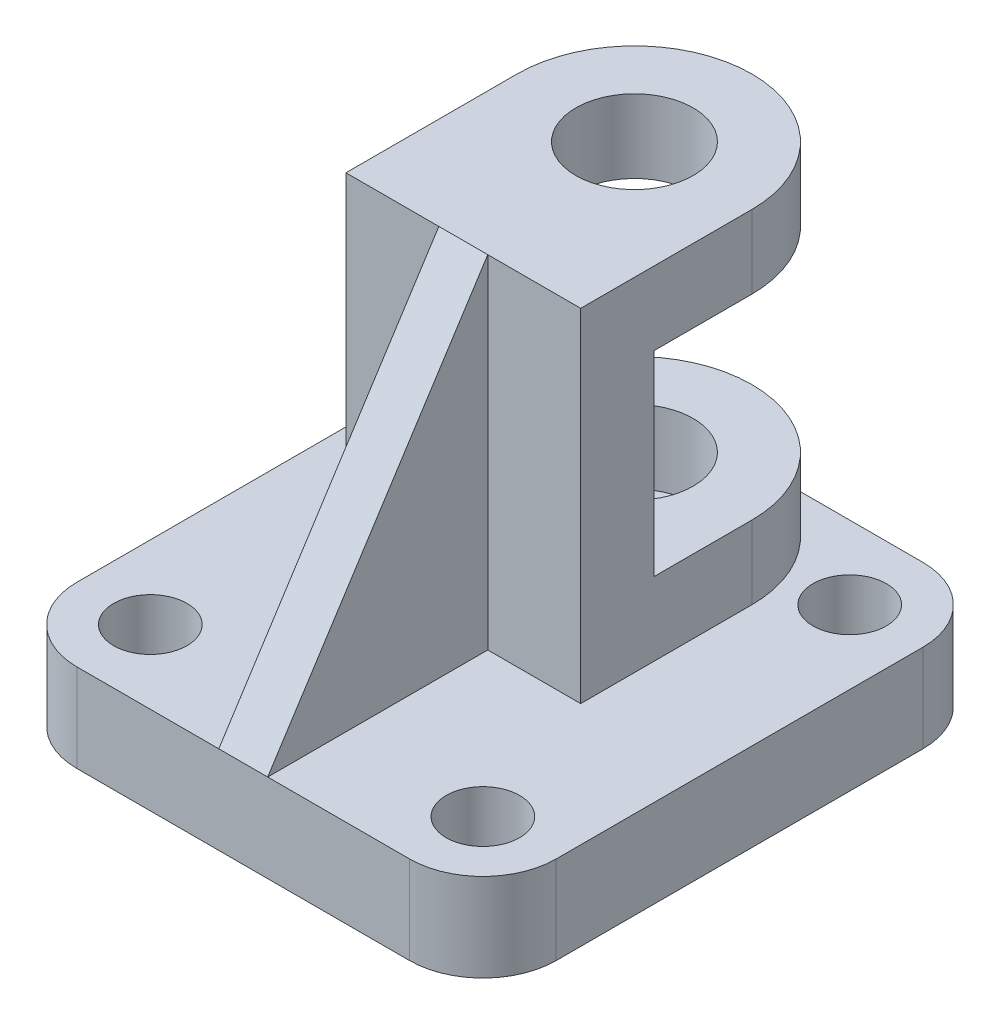
ISO-10303-21;
HEADER;
FILE_DESCRIPTION(('STEP AP214'),'2;1');
FILE_NAME('part.step','',(''),(''),'','','');
FILE_SCHEMA(('AUTOMOTIVE_DESIGN { 1 0 10303 214 1 1 1 1 }'));
ENDSEC;
DATA;
#1=APPLICATION_CONTEXT('core data for automotive mechanical design processes');
#2=APPLICATION_PROTOCOL_DEFINITION('international standard','automotive_design',2000,#1);
#3=PRODUCT_CONTEXT('',#1,'mechanical');
#4=PRODUCT('Part','Part','',(#3));
#5=PRODUCT_RELATED_PRODUCT_CATEGORY('part','',(#4));
#6=PRODUCT_DEFINITION_FORMATION('','',#4);
#7=PRODUCT_DEFINITION_CONTEXT('part definition',#1,'design');
#8=PRODUCT_DEFINITION('design','',#6,#7);
#9=PRODUCT_DEFINITION_SHAPE('','',#8);
#10=(LENGTH_UNIT() NAMED_UNIT(*) SI_UNIT(.MILLI.,.METRE.));
#11=(NAMED_UNIT(*) PLANE_ANGLE_UNIT() SI_UNIT($,.RADIAN.));
#12=(NAMED_UNIT(*) SI_UNIT($,.STERADIAN.) SOLID_ANGLE_UNIT());
#13=UNCERTAINTY_MEASURE_WITH_UNIT(LENGTH_MEASURE(1.E-05),#10,'distance_accuracy_value','');
#14=(GEOMETRIC_REPRESENTATION_CONTEXT(3) GLOBAL_UNCERTAINTY_ASSIGNED_CONTEXT((#13)) GLOBAL_UNIT_ASSIGNED_CONTEXT((#10,
#11,#12)) REPRESENTATION_CONTEXT('',''));
#15=CARTESIAN_POINT('',(0.,0.,0.));
#16=DIRECTION('',(0.,0.,1.));
#17=DIRECTION('',(1.,0.,0.));
#18=AXIS2_PLACEMENT_3D('',#15,#16,#17);
#19=CARTESIAN_POINT('',(0.,0.,7.5));
#20=DIRECTION('',(0.,0.,-1.));
#21=DIRECTION('',(-1.,0.,0.));
#22=AXIS2_PLACEMENT_3D('',#19,#20,#21);
#23=PLANE('',#22);
#24=DIRECTION('',(1.,0.,0.));
#25=VECTOR('',#24,1.);
#26=CARTESIAN_POINT('',(-24.,18.,7.5));
#27=LINE('',#26,#25);
#28=CARTESIAN_POINT('',(-24.,18.,7.5));
#29=VERTEX_POINT('',#28);
#30=CARTESIAN_POINT('',(-5.,18.,7.5));
#31=VERTEX_POINT('',#30);
#32=EDGE_CURVE('E251',#29,#31,#27,.T.);
#33=ORIENTED_EDGE('',*,*,#32,.T.);
#34=DIRECTION('',(0.,-1.,0.));
#35=VECTOR('',#34,1.);
#36=CARTESIAN_POINT('',(-5.,0.,7.5));
#37=LINE('',#36,#35);
#38=CARTESIAN_POINT('',(-5.,88.,7.5));
#39=VERTEX_POINT('',#38);
#40=EDGE_CURVE('E235',#39,#31,#37,.T.);
#41=ORIENTED_EDGE('',*,*,#40,.F.);
#42=DIRECTION('',(-1.,0.,0.));
#43=VECTOR('',#42,1.);
#44=CARTESIAN_POINT('',(-24.,88.,7.5));
#45=LINE('',#44,#43);
#46=CARTESIAN_POINT('',(-24.,88.,7.5));
#47=VERTEX_POINT('',#46);
#48=EDGE_CURVE('E256',#39,#47,#45,.T.);
#49=ORIENTED_EDGE('',*,*,#48,.T.);
#50=DIRECTION('',(0.,-1.,0.));
#51=VECTOR('',#50,1.);
#52=CARTESIAN_POINT('',(-24.,18.,7.5));
#53=LINE('',#52,#51);
#54=EDGE_CURVE('E248',#47,#29,#53,.T.);
#55=ORIENTED_EDGE('',*,*,#54,.T.);
#56=EDGE_LOOP('',(#33,#41,#49,#55));
#57=FACE_BOUND('',#56,.T.);
#58=ADVANCED_FACE('F41',(#57),#23,.F.);
#59=CARTESIAN_POINT('',(-34.,18.,37.5));
#60=DIRECTION('',(0.,-1.,0.));
#61=DIRECTION('',(0.,0.,-1.));
#62=AXIS2_PLACEMENT_3D('',#59,#60,#61);
#63=PLANE('',#62);
#64=CARTESIAN_POINT('',(34.,18.,37.5));
#65=DIRECTION('',(0.,1.,0.));
#66=DIRECTION('',(0.,0.,1.));
#67=AXIS2_PLACEMENT_3D('',#64,#65,#66);
#68=CIRCLE('',#67,7.5);
#69=CARTESIAN_POINT('',(34.,18.,45.));
#70=VERTEX_POINT('',#69);
#71=EDGE_CURVE('E275',#70,#70,#68,.T.);
#72=ORIENTED_EDGE('',*,*,#71,.F.);
#73=EDGE_LOOP('',(#72));
#74=FACE_BOUND('',#73,.T.);
#75=CARTESIAN_POINT('',(34.,18.,-37.5));
#76=DIRECTION('',(0.,1.,0.));
#77=DIRECTION('',(0.,0.,1.));
#78=AXIS2_PLACEMENT_3D('',#75,#76,#77);
#79=CIRCLE('',#78,7.5);
#80=CARTESIAN_POINT('',(34.,18.,-30.));
#81=VERTEX_POINT('',#80);
#82=EDGE_CURVE('E279',#81,#81,#79,.T.);
#83=ORIENTED_EDGE('',*,*,#82,.F.);
#84=EDGE_LOOP('',(#83));
#85=FACE_BOUND('',#84,.T.);
#86=DIRECTION('',(0.,0.,-1.));
#87=VECTOR('',#86,1.);
#88=CARTESIAN_POINT('',(-24.,18.,7.5));
#89=LINE('',#88,#87);
#90=CARTESIAN_POINT('',(-24.,18.,-27.5));
#91=VERTEX_POINT('',#90);
#92=EDGE_CURVE('E57',#29,#91,#89,.T.);
#93=ORIENTED_EDGE('',*,*,#92,.T.);
#94=CARTESIAN_POINT('',(0.,18.,-27.5));
#95=DIRECTION('',(0.,1.,0.));
#96=DIRECTION('',(0.,0.,1.));
#97=AXIS2_PLACEMENT_3D('',#94,#95,#96);
#98=CIRCLE('',#97,24.);
#99=CARTESIAN_POINT('',(24.,18.,-27.5));
#100=VERTEX_POINT('',#99);
#101=EDGE_CURVE('E178',#91,#100,#98,.F.);
#102=ORIENTED_EDGE('',*,*,#101,.T.);
#103=DIRECTION('',(0.,0.,-1.));
#104=VECTOR('',#103,1.);
#105=CARTESIAN_POINT('',(24.,18.,7.5));
#106=LINE('',#105,#104);
#107=CARTESIAN_POINT('',(24.,18.,7.5));
#108=VERTEX_POINT('',#107);
#109=EDGE_CURVE('E61',#108,#100,#106,.T.);
#110=ORIENTED_EDGE('',*,*,#109,.F.);
#111=CARTESIAN_POINT('',(5.,18.,7.5));
#112=VERTEX_POINT('',#111);
#113=EDGE_CURVE('E253',#112,#108,#27,.T.);
#114=ORIENTED_EDGE('',*,*,#113,.F.);
#115=DIRECTION('',(0.,0.,1.));
#116=VECTOR('',#115,1.);
#117=CARTESIAN_POINT('',(5.,18.,37.5));
#118=LINE('',#117,#116);
#119=CARTESIAN_POINT('',(5.,18.,52.5));
#120=VERTEX_POINT('',#119);
#121=EDGE_CURVE('E245',#112,#120,#118,.T.);
#122=ORIENTED_EDGE('',*,*,#121,.T.);
#123=DIRECTION('',(1.,0.,0.));
#124=VECTOR('',#123,1.);
#125=CARTESIAN_POINT('',(-33.9999999999999,18.,52.5));
#126=LINE('',#125,#124);
#127=CARTESIAN_POINT('',(33.9999999999999,18.,52.5));
#128=VERTEX_POINT('',#127);
#129=EDGE_CURVE('E296',#120,#128,#126,.T.);
#130=ORIENTED_EDGE('',*,*,#129,.T.);
#131=CARTESIAN_POINT('',(34.,18.,37.5));
#132=DIRECTION('',(0.,1.,0.));
#133=DIRECTION('',(0.,0.,1.));
#134=AXIS2_PLACEMENT_3D('',#131,#132,#133);
#135=CIRCLE('',#134,15.);
#136=CARTESIAN_POINT('',(49.,18.,37.4999999999999));
#137=VERTEX_POINT('',#136);
#138=EDGE_CURVE('E303',#128,#137,#135,.T.);
#139=ORIENTED_EDGE('',*,*,#138,.T.);
#140=DIRECTION('',(0.,0.,-1.));
#141=VECTOR('',#140,1.);
#142=CARTESIAN_POINT('',(49.,18.,37.4999999999999));
#143=LINE('',#142,#141);
#144=CARTESIAN_POINT('',(49.,18.,-37.4999999999999));
#145=VERTEX_POINT('',#144);
#146=EDGE_CURVE('E308',#137,#145,#143,.T.);
#147=ORIENTED_EDGE('',*,*,#146,.T.);
#148=CARTESIAN_POINT('',(34.,18.,-37.5));
#149=DIRECTION('',(0.,1.,0.));
#150=DIRECTION('',(0.,0.,-1.));
#151=AXIS2_PLACEMENT_3D('',#148,#149,#150);
#152=CIRCLE('',#151,15.);
#153=CARTESIAN_POINT('',(33.9999999999999,18.,-52.5));
#154=VERTEX_POINT('',#153);
#155=EDGE_CURVE('E306',#145,#154,#152,.T.);
#156=ORIENTED_EDGE('',*,*,#155,.T.);
#157=DIRECTION('',(-1.,0.,0.));
#158=VECTOR('',#157,1.);
#159=CARTESIAN_POINT('',(-33.9999999999999,18.,-52.5));
#160=LINE('',#159,#158);
#161=CARTESIAN_POINT('',(-33.9999999999999,18.,-52.5));
#162=VERTEX_POINT('',#161);
#163=EDGE_CURVE('E309',#154,#162,#160,.T.);
#164=ORIENTED_EDGE('',*,*,#163,.T.);
#165=CARTESIAN_POINT('',(-34.,18.,-37.5));
#166=DIRECTION('',(0.,1.,0.));
#167=DIRECTION('',(0.,0.,-1.));
#168=AXIS2_PLACEMENT_3D('',#165,#166,#167);
#169=CIRCLE('',#168,15.);
#170=CARTESIAN_POINT('',(-49.,18.,-37.4999999999999));
#171=VERTEX_POINT('',#170);
#172=EDGE_CURVE('E315',#162,#171,#169,.T.);
#173=ORIENTED_EDGE('',*,*,#172,.T.);
#174=DIRECTION('',(0.,0.,1.));
#175=VECTOR('',#174,1.);
#176=CARTESIAN_POINT('',(-49.,18.,37.4999999999999));
#177=LINE('',#176,#175);
#178=CARTESIAN_POINT('',(-49.,18.,37.4999999999999));
#179=VERTEX_POINT('',#178);
#180=EDGE_CURVE('E314',#171,#179,#177,.T.);
#181=ORIENTED_EDGE('',*,*,#180,.T.);
#182=CARTESIAN_POINT('',(-34.,18.,37.5));
#183=DIRECTION('',(0.,1.,0.));
#184=DIRECTION('',(0.,0.,-1.));
#185=AXIS2_PLACEMENT_3D('',#182,#183,#184);
#186=CIRCLE('',#185,15.);
#187=CARTESIAN_POINT('',(-33.9999999999999,18.,52.5));
#188=VERTEX_POINT('',#187);
#189=EDGE_CURVE('E297',#179,#188,#186,.T.);
#190=ORIENTED_EDGE('',*,*,#189,.T.);
#191=CARTESIAN_POINT('',(-5.,18.,52.5));
#192=VERTEX_POINT('',#191);
#193=EDGE_CURVE('E301',#188,#192,#126,.T.);
#194=ORIENTED_EDGE('',*,*,#193,.T.);
#195=DIRECTION('',(0.,0.,1.));
#196=VECTOR('',#195,1.);
#197=CARTESIAN_POINT('',(-5.,18.,37.5));
#198=LINE('',#197,#196);
#199=EDGE_CURVE('E236',#31,#192,#198,.T.);
#200=ORIENTED_EDGE('',*,*,#199,.F.);
#201=ORIENTED_EDGE('',*,*,#32,.F.);
#202=EDGE_LOOP('',(#93,#102,#110,#114,#122,#130,#139,#147,#156,#164,#173,#181,#190,#194,#200,#201));
#203=FACE_BOUND('',#202,.T.);
#204=CARTESIAN_POINT('',(-34.,18.,37.5));
#205=DIRECTION('',(0.,1.,0.));
#206=DIRECTION('',(0.,0.,1.));
#207=AXIS2_PLACEMENT_3D('',#204,#205,#206);
#208=CIRCLE('',#207,7.5);
#209=CARTESIAN_POINT('',(-34.,18.,45.));
#210=VERTEX_POINT('',#209);
#211=EDGE_CURVE('E283',#210,#210,#208,.T.);
#212=ORIENTED_EDGE('',*,*,#211,.F.);
#213=EDGE_LOOP('',(#212));
#214=FACE_BOUND('',#213,.T.);
#215=CARTESIAN_POINT('',(-34.,18.,-37.5));
#216=DIRECTION('',(0.,1.,0.));
#217=DIRECTION('',(0.,0.,1.));
#218=AXIS2_PLACEMENT_3D('',#215,#216,#217);
#219=CIRCLE('',#218,7.5);
#220=CARTESIAN_POINT('',(-34.,18.,-30.));
#221=VERTEX_POINT('',#220);
#222=EDGE_CURVE('E282',#221,#221,#219,.T.);
#223=ORIENTED_EDGE('',*,*,#222,.F.);
#224=EDGE_LOOP('',(#223));
#225=FACE_BOUND('',#224,.T.);
#226=ADVANCED_FACE('F378',(#74,#85,#203,#214,#225),#63,.F.);
#227=CARTESIAN_POINT('',(-34.,18.,37.5));
#228=DIRECTION('',(0.,-1.,0.));
#229=DIRECTION('',(0.,0.,-1.));
#230=AXIS2_PLACEMENT_3D('',#227,#228,#229);
#231=CYLINDRICAL_SURFACE('',#230,15.);
#232=CARTESIAN_POINT('',(-34.,0.,37.5));
#233=DIRECTION('',(0.,1.,0.));
#234=DIRECTION('',(0.,0.,-1.));
#235=AXIS2_PLACEMENT_3D('',#232,#233,#234);
#236=CIRCLE('',#235,15.);
#237=CARTESIAN_POINT('',(-49.,0.,37.4999999999999));
#238=VERTEX_POINT('',#237);
#239=CARTESIAN_POINT('',(-33.9999999999999,0.,52.5));
#240=VERTEX_POINT('',#239);
#241=EDGE_CURVE('E291',#238,#240,#236,.T.);
#242=ORIENTED_EDGE('',*,*,#241,.T.);
#243=DIRECTION('',(0.,-1.,0.));
#244=VECTOR('',#243,1.);
#245=CARTESIAN_POINT('',(-33.9999999999999,18.,52.5));
#246=LINE('',#245,#244);
#247=EDGE_CURVE('E47',#188,#240,#246,.T.);
#248=ORIENTED_EDGE('',*,*,#247,.F.);
#249=ORIENTED_EDGE('',*,*,#189,.F.);
#250=DIRECTION('',(0.,-1.,0.));
#251=VECTOR('',#250,1.);
#252=CARTESIAN_POINT('',(-49.,18.,37.4999999999999));
#253=LINE('',#252,#251);
#254=EDGE_CURVE('E316',#179,#238,#253,.T.);
#255=ORIENTED_EDGE('',*,*,#254,.T.);
#256=EDGE_LOOP('',(#242,#248,#249,#255));
#257=FACE_BOUND('',#256,.T.);
#258=ADVANCED_FACE('F43',(#257),#231,.T.);
#259=CARTESIAN_POINT('',(-33.9999999999999,18.,52.5));
#260=DIRECTION('',(0.,0.,-1.));
#261=DIRECTION('',(-1.,0.,0.));
#262=AXIS2_PLACEMENT_3D('',#259,#260,#261);
#263=PLANE('',#262);
#264=ORIENTED_EDGE('',*,*,#129,.F.);
#265=DIRECTION('',(1.,0.,0.));
#266=VECTOR('',#265,1.);
#267=CARTESIAN_POINT('',(-33.9999999999999,18.,52.5));
#268=LINE('',#267,#266);
#269=EDGE_CURVE('E243',#192,#120,#268,.T.);
#270=ORIENTED_EDGE('',*,*,#269,.F.);
#271=ORIENTED_EDGE('',*,*,#193,.F.);
#272=ORIENTED_EDGE('',*,*,#247,.T.);
#273=DIRECTION('',(1.,0.,0.));
#274=VECTOR('',#273,1.);
#275=CARTESIAN_POINT('',(-33.9999999999999,0.,52.5));
#276=LINE('',#275,#274);
#277=CARTESIAN_POINT('',(33.9999999999999,0.,52.5));
#278=VERTEX_POINT('',#277);
#279=EDGE_CURVE('E317',#240,#278,#276,.T.);
#280=ORIENTED_EDGE('',*,*,#279,.T.);
#281=DIRECTION('',(0.,-1.,0.));
#282=VECTOR('',#281,1.);
#283=CARTESIAN_POINT('',(33.9999999999999,18.,52.5));
#284=LINE('',#283,#282);
#285=EDGE_CURVE('E349',#128,#278,#284,.T.);
#286=ORIENTED_EDGE('',*,*,#285,.F.);
#287=EDGE_LOOP('',(#264,#270,#271,#272,#280,#286));
#288=FACE_BOUND('',#287,.T.);
#289=ADVANCED_FACE('F353',(#288),#263,.F.);
#290=CARTESIAN_POINT('',(34.,18.,37.5));
#291=DIRECTION('',(0.,-1.,0.));
#292=DIRECTION('',(0.,0.,-1.));
#293=AXIS2_PLACEMENT_3D('',#290,#291,#292);
#294=CYLINDRICAL_SURFACE('',#293,15.);
#295=CARTESIAN_POINT('',(34.,0.,37.5));
#296=DIRECTION('',(0.,1.,0.));
#297=DIRECTION('',(0.,0.,1.));
#298=AXIS2_PLACEMENT_3D('',#295,#296,#297);
#299=CIRCLE('',#298,15.);
#300=CARTESIAN_POINT('',(49.,0.,37.4999999999999));
#301=VERTEX_POINT('',#300);
#302=EDGE_CURVE('E321',#278,#301,#299,.T.);
#303=ORIENTED_EDGE('',*,*,#302,.T.);
#304=DIRECTION('',(0.,-1.,0.));
#305=VECTOR('',#304,1.);
#306=CARTESIAN_POINT('',(49.,18.,37.4999999999999));
#307=LINE('',#306,#305);
#308=EDGE_CURVE('E347',#137,#301,#307,.T.);
#309=ORIENTED_EDGE('',*,*,#308,.F.);
#310=ORIENTED_EDGE('',*,*,#138,.F.);
#311=ORIENTED_EDGE('',*,*,#285,.T.);
#312=EDGE_LOOP('',(#303,#309,#310,#311));
#313=FACE_BOUND('',#312,.T.);
#314=ADVANCED_FACE('F371',(#313),#294,.T.);
#315=CARTESIAN_POINT('',(49.,18.,37.4999999999999));
#316=DIRECTION('',(-1.,0.,0.));
#317=DIRECTION('',(0.,0.,1.));
#318=AXIS2_PLACEMENT_3D('',#315,#316,#317);
#319=PLANE('',#318);
#320=DIRECTION('',(0.,0.,-1.));
#321=VECTOR('',#320,1.);
#322=CARTESIAN_POINT('',(49.,0.,37.4999999999999));
#323=LINE('',#322,#321);
#324=CARTESIAN_POINT('',(49.,0.,-37.4999999999999));
#325=VERTEX_POINT('',#324);
#326=EDGE_CURVE('E323',#301,#325,#323,.T.);
#327=ORIENTED_EDGE('',*,*,#326,.T.);
#328=DIRECTION('',(0.,-1.,0.));
#329=VECTOR('',#328,1.);
#330=CARTESIAN_POINT('',(49.,18.,-37.4999999999999));
#331=LINE('',#330,#329);
#332=EDGE_CURVE('E344',#145,#325,#331,.T.);
#333=ORIENTED_EDGE('',*,*,#332,.F.);
#334=ORIENTED_EDGE('',*,*,#146,.F.);
#335=ORIENTED_EDGE('',*,*,#308,.T.);
#336=EDGE_LOOP('',(#327,#333,#334,#335));
#337=FACE_BOUND('',#336,.T.);
#338=ADVANCED_FACE('F374',(#337),#319,.F.);
#339=CARTESIAN_POINT('',(34.,18.,-37.5));
#340=DIRECTION('',(0.,-1.,0.));
#341=DIRECTION('',(0.,0.,-1.));
#342=AXIS2_PLACEMENT_3D('',#339,#340,#341);
#343=CYLINDRICAL_SURFACE('',#342,15.);
#344=CARTESIAN_POINT('',(34.,0.,-37.5));
#345=DIRECTION('',(0.,1.,0.));
#346=DIRECTION('',(0.,0.,-1.));
#347=AXIS2_PLACEMENT_3D('',#344,#345,#346);
#348=CIRCLE('',#347,15.);
#349=CARTESIAN_POINT('',(33.9999999999999,0.,-52.5));
#350=VERTEX_POINT('',#349);
#351=EDGE_CURVE('E324',#325,#350,#348,.T.);
#352=ORIENTED_EDGE('',*,*,#351,.T.);
#353=DIRECTION('',(0.,-1.,0.));
#354=VECTOR('',#353,1.);
#355=CARTESIAN_POINT('',(33.9999999999999,18.,-52.5));
#356=LINE('',#355,#354);
#357=EDGE_CURVE('E338',#154,#350,#356,.T.);
#358=ORIENTED_EDGE('',*,*,#357,.F.);
#359=ORIENTED_EDGE('',*,*,#155,.F.);
#360=ORIENTED_EDGE('',*,*,#332,.T.);
#361=EDGE_LOOP('',(#352,#358,#359,#360));
#362=FACE_BOUND('',#361,.T.);
#363=ADVANCED_FACE('F480',(#362),#343,.T.);
#364=CARTESIAN_POINT('',(-33.9999999999999,18.,-52.5));
#365=DIRECTION('',(0.,0.,1.));
#366=DIRECTION('',(1.,0.,0.));
#367=AXIS2_PLACEMENT_3D('',#364,#365,#366);
#368=PLANE('',#367);
#369=DIRECTION('',(-1.,0.,0.));
#370=VECTOR('',#369,1.);
#371=CARTESIAN_POINT('',(-33.9999999999999,0.,-52.5));
#372=LINE('',#371,#370);
#373=CARTESIAN_POINT('',(-33.9999999999999,0.,-52.5));
#374=VERTEX_POINT('',#373);
#375=EDGE_CURVE('E330',#350,#374,#372,.T.);
#376=ORIENTED_EDGE('',*,*,#375,.T.);
#377=DIRECTION('',(0.,-1.,0.));
#378=VECTOR('',#377,1.);
#379=CARTESIAN_POINT('',(-33.9999999999999,18.,-52.5));
#380=LINE('',#379,#378);
#381=EDGE_CURVE('E339',#162,#374,#380,.T.);
#382=ORIENTED_EDGE('',*,*,#381,.F.);
#383=ORIENTED_EDGE('',*,*,#163,.F.);
#384=ORIENTED_EDGE('',*,*,#357,.T.);
#385=EDGE_LOOP('',(#376,#382,#383,#384));
#386=FACE_BOUND('',#385,.T.);
#387=ADVANCED_FACE('F471',(#386),#368,.F.);
#388=CARTESIAN_POINT('',(-34.,18.,-37.5));
#389=DIRECTION('',(0.,-1.,0.));
#390=DIRECTION('',(0.,0.,-1.));
#391=AXIS2_PLACEMENT_3D('',#388,#389,#390);
#392=CYLINDRICAL_SURFACE('',#391,15.);
#393=CARTESIAN_POINT('',(-34.,0.,-37.5));
#394=DIRECTION('',(0.,1.,0.));
#395=DIRECTION('',(0.,0.,-1.));
#396=AXIS2_PLACEMENT_3D('',#393,#394,#395);
#397=CIRCLE('',#396,15.);
#398=CARTESIAN_POINT('',(-49.,0.,-37.4999999999999));
#399=VERTEX_POINT('',#398);
#400=EDGE_CURVE('E328',#374,#399,#397,.T.);
#401=ORIENTED_EDGE('',*,*,#400,.T.);
#402=DIRECTION('',(0.,-1.,0.));
#403=VECTOR('',#402,1.);
#404=CARTESIAN_POINT('',(-49.,18.,-37.4999999999999));
#405=LINE('',#404,#403);
#406=EDGE_CURVE('E331',#171,#399,#405,.T.);
#407=ORIENTED_EDGE('',*,*,#406,.F.);
#408=ORIENTED_EDGE('',*,*,#172,.F.);
#409=ORIENTED_EDGE('',*,*,#381,.T.);
#410=EDGE_LOOP('',(#401,#407,#408,#409));
#411=FACE_BOUND('',#410,.T.);
#412=ADVANCED_FACE('F468',(#411),#392,.T.);
#413=CARTESIAN_POINT('',(-49.,18.,37.4999999999999));
#414=DIRECTION('',(1.,0.,0.));
#415=DIRECTION('',(0.,0.,-1.));
#416=AXIS2_PLACEMENT_3D('',#413,#414,#415);
#417=PLANE('',#416);
#418=DIRECTION('',(0.,0.,1.));
#419=VECTOR('',#418,1.);
#420=CARTESIAN_POINT('',(-49.,0.,37.4999999999999));
#421=LINE('',#420,#419);
#422=EDGE_CURVE('E298',#399,#238,#421,.T.);
#423=ORIENTED_EDGE('',*,*,#422,.T.);
#424=ORIENTED_EDGE('',*,*,#254,.F.);
#425=ORIENTED_EDGE('',*,*,#180,.F.);
#426=ORIENTED_EDGE('',*,*,#406,.T.);
#427=EDGE_LOOP('',(#423,#424,#425,#426));
#428=FACE_BOUND('',#427,.T.);
#429=ADVANCED_FACE('F466',(#428),#417,.F.);
#430=CARTESIAN_POINT('',(-34.,0.,37.5));
#431=DIRECTION('',(0.,-1.,0.));
#432=DIRECTION('',(0.,0.,-1.));
#433=AXIS2_PLACEMENT_3D('',#430,#431,#432);
#434=PLANE('',#433);
#435=ORIENTED_EDGE('',*,*,#302,.F.);
#436=ORIENTED_EDGE('',*,*,#279,.F.);
#437=ORIENTED_EDGE('',*,*,#241,.F.);
#438=ORIENTED_EDGE('',*,*,#422,.F.);
#439=ORIENTED_EDGE('',*,*,#400,.F.);
#440=ORIENTED_EDGE('',*,*,#375,.F.);
#441=ORIENTED_EDGE('',*,*,#351,.F.);
#442=ORIENTED_EDGE('',*,*,#326,.F.);
#443=EDGE_LOOP('',(#435,#436,#437,#438,#439,#440,#441,#442));
#444=FACE_BOUND('',#443,.T.);
#445=CARTESIAN_POINT('',(34.,0.,-37.5));
#446=DIRECTION('',(0.,1.,0.));
#447=DIRECTION('',(0.,0.,1.));
#448=AXIS2_PLACEMENT_3D('',#445,#446,#447);
#449=CIRCLE('',#448,7.5);
#450=CARTESIAN_POINT('',(34.,0.,-30.));
#451=VERTEX_POINT('',#450);
#452=EDGE_CURVE('E284',#451,#451,#449,.T.);
#453=ORIENTED_EDGE('',*,*,#452,.T.);
#454=EDGE_LOOP('',(#453));
#455=FACE_BOUND('',#454,.T.);
#456=CARTESIAN_POINT('',(34.,0.,37.5));
#457=DIRECTION('',(0.,1.,0.));
#458=DIRECTION('',(0.,0.,1.));
#459=AXIS2_PLACEMENT_3D('',#456,#457,#458);
#460=CIRCLE('',#459,7.5);
#461=CARTESIAN_POINT('',(34.,0.,45.));
#462=VERTEX_POINT('',#461);
#463=EDGE_CURVE('E271',#462,#462,#460,.T.);
#464=ORIENTED_EDGE('',*,*,#463,.T.);
#465=EDGE_LOOP('',(#464));
#466=FACE_BOUND('',#465,.T.);
#467=CARTESIAN_POINT('',(-34.,0.,-37.5));
#468=DIRECTION('',(0.,1.,0.));
#469=DIRECTION('',(0.,0.,1.));
#470=AXIS2_PLACEMENT_3D('',#467,#468,#469);
#471=CIRCLE('',#470,7.5);
#472=CARTESIAN_POINT('',(-34.,0.,-30.));
#473=VERTEX_POINT('',#472);
#474=EDGE_CURVE('E290',#473,#473,#471,.T.);
#475=ORIENTED_EDGE('',*,*,#474,.T.);
#476=EDGE_LOOP('',(#475));
#477=FACE_BOUND('',#476,.T.);
#478=CARTESIAN_POINT('',(-34.,0.,37.5));
#479=DIRECTION('',(0.,1.,0.));
#480=DIRECTION('',(0.,0.,1.));
#481=AXIS2_PLACEMENT_3D('',#478,#479,#480);
#482=CIRCLE('',#481,7.5);
#483=CARTESIAN_POINT('',(-34.,0.,45.));
#484=VERTEX_POINT('',#483);
#485=EDGE_CURVE('E274',#484,#484,#482,.T.);
#486=ORIENTED_EDGE('',*,*,#485,.T.);
#487=EDGE_LOOP('',(#486));
#488=FACE_BOUND('',#487,.T.);
#489=ADVANCED_FACE('F365',(#444,#455,#466,#477,#488),#434,.T.);
#490=CARTESIAN_POINT('',(-34.,0.,-37.5));
#491=DIRECTION('',(0.,1.,0.));
#492=DIRECTION('',(0.,0.,1.));
#493=AXIS2_PLACEMENT_3D('',#490,#491,#492);
#494=CYLINDRICAL_SURFACE('',#493,7.5);
#495=ORIENTED_EDGE('',*,*,#474,.F.);
#496=EDGE_LOOP('',(#495));
#497=FACE_BOUND('',#496,.T.);
#498=ORIENTED_EDGE('',*,*,#222,.T.);
#499=EDGE_LOOP('',(#498));
#500=FACE_BOUND('',#499,.T.);
#501=ADVANCED_FACE('F464',(#497,#500),#494,.F.);
#502=CARTESIAN_POINT('',(34.,0.,37.5));
#503=DIRECTION('',(0.,1.,0.));
#504=DIRECTION('',(0.,0.,1.));
#505=AXIS2_PLACEMENT_3D('',#502,#503,#504);
#506=CYLINDRICAL_SURFACE('',#505,7.5);
#507=ORIENTED_EDGE('',*,*,#463,.F.);
#508=EDGE_LOOP('',(#507));
#509=FACE_BOUND('',#508,.T.);
#510=ORIENTED_EDGE('',*,*,#71,.T.);
#511=EDGE_LOOP('',(#510));
#512=FACE_BOUND('',#511,.T.);
#513=ADVANCED_FACE('F528',(#509,#512),#506,.F.);
#514=CARTESIAN_POINT('',(-34.,0.,37.5));
#515=DIRECTION('',(0.,1.,0.));
#516=DIRECTION('',(0.,0.,1.));
#517=AXIS2_PLACEMENT_3D('',#514,#515,#516);
#518=CYLINDRICAL_SURFACE('',#517,7.5);
#519=ORIENTED_EDGE('',*,*,#485,.F.);
#520=EDGE_LOOP('',(#519));
#521=FACE_BOUND('',#520,.T.);
#522=ORIENTED_EDGE('',*,*,#211,.T.);
#523=EDGE_LOOP('',(#522));
#524=FACE_BOUND('',#523,.T.);
#525=ADVANCED_FACE('F534',(#521,#524),#518,.F.);
#526=CARTESIAN_POINT('',(34.,0.,-37.5));
#527=DIRECTION('',(0.,1.,0.));
#528=DIRECTION('',(0.,0.,1.));
#529=AXIS2_PLACEMENT_3D('',#526,#527,#528);
#530=CYLINDRICAL_SURFACE('',#529,7.5);
#531=ORIENTED_EDGE('',*,*,#452,.F.);
#532=EDGE_LOOP('',(#531));
#533=FACE_BOUND('',#532,.T.);
#534=ORIENTED_EDGE('',*,*,#82,.T.);
#535=EDGE_LOOP('',(#534));
#536=FACE_BOUND('',#535,.T.);
#537=ADVANCED_FACE('F545',(#533,#536),#530,.F.);
#538=CARTESIAN_POINT('',(-24.,18.,7.5));
#539=DIRECTION('',(1.,0.,0.));
#540=DIRECTION('',(0.,0.,-1.));
#541=AXIS2_PLACEMENT_3D('',#538,#539,#540);
#542=PLANE('',#541);
#543=ORIENTED_EDGE('',*,*,#92,.F.);
#544=ORIENTED_EDGE('',*,*,#54,.F.);
#545=DIRECTION('',(0.,0.,-1.));
#546=VECTOR('',#545,1.);
#547=CARTESIAN_POINT('',(-24.,88.,7.5));
#548=LINE('',#547,#546);
#549=CARTESIAN_POINT('',(-24.,88.,-27.5));
#550=VERTEX_POINT('',#549);
#551=EDGE_CURVE('E265',#47,#550,#548,.T.);
#552=ORIENTED_EDGE('',*,*,#551,.T.);
#553=DIRECTION('',(0.,1.,0.));
#554=VECTOR('',#553,1.);
#555=CARTESIAN_POINT('',(-24.,73.,-27.5));
#556=LINE('',#555,#554);
#557=CARTESIAN_POINT('',(-24.,73.,-27.5));
#558=VERTEX_POINT('',#557);
#559=EDGE_CURVE('E227',#558,#550,#556,.T.);
#560=ORIENTED_EDGE('',*,*,#559,.F.);
#561=DIRECTION('',(0.,0.,1.));
#562=VECTOR('',#561,1.);
#563=CARTESIAN_POINT('',(-24.,73.,7.5));
#564=LINE('',#563,#562);
#565=CARTESIAN_POINT('',(-24.,73.,-7.5));
#566=VERTEX_POINT('',#565);
#567=EDGE_CURVE('E222',#558,#566,#564,.T.);
#568=ORIENTED_EDGE('',*,*,#567,.T.);
#569=DIRECTION('',(0.,-1.,0.));
#570=VECTOR('',#569,1.);
#571=CARTESIAN_POINT('',(-24.,18.,-7.5));
#572=LINE('',#571,#570);
#573=CARTESIAN_POINT('',(-24.,33.,-7.5));
#574=VERTEX_POINT('',#573);
#575=EDGE_CURVE('E196',#566,#574,#572,.T.);
#576=ORIENTED_EDGE('',*,*,#575,.T.);
#577=DIRECTION('',(0.,0.,-1.));
#578=VECTOR('',#577,1.);
#579=CARTESIAN_POINT('',(-24.,33.,0.));
#580=LINE('',#579,#578);
#581=CARTESIAN_POINT('',(-24.,33.,-27.5));
#582=VERTEX_POINT('',#581);
#583=EDGE_CURVE('E186',#574,#582,#580,.T.);
#584=ORIENTED_EDGE('',*,*,#583,.T.);
#585=DIRECTION('',(0.,-1.,0.));
#586=VECTOR('',#585,1.);
#587=CARTESIAN_POINT('',(-24.,33.,-27.5));
#588=LINE('',#587,#586);
#589=EDGE_CURVE('E175',#582,#91,#588,.T.);
#590=ORIENTED_EDGE('',*,*,#589,.T.);
#591=EDGE_LOOP('',(#543,#544,#552,#560,#568,#576,#584,#590));
#592=FACE_BOUND('',#591,.T.);
#593=ADVANCED_FACE('F195',(#592),#542,.F.);
#594=CARTESIAN_POINT('',(24.,18.,7.5));
#595=DIRECTION('',(-1.,0.,0.));
#596=DIRECTION('',(0.,0.,1.));
#597=AXIS2_PLACEMENT_3D('',#594,#595,#596);
#598=PLANE('',#597);
#599=ORIENTED_EDGE('',*,*,#109,.T.);
#600=DIRECTION('',(0.,-1.,0.));
#601=VECTOR('',#600,1.);
#602=CARTESIAN_POINT('',(24.,33.,-27.5));
#603=LINE('',#602,#601);
#604=CARTESIAN_POINT('',(24.,33.,-27.5));
#605=VERTEX_POINT('',#604);
#606=EDGE_CURVE('E181',#605,#100,#603,.T.);
#607=ORIENTED_EDGE('',*,*,#606,.F.);
#608=DIRECTION('',(0.,0.,1.));
#609=VECTOR('',#608,1.);
#610=CARTESIAN_POINT('',(24.,33.,0.));
#611=LINE('',#610,#609);
#612=CARTESIAN_POINT('',(24.,33.,-7.5));
#613=VERTEX_POINT('',#612);
#614=EDGE_CURVE('E191',#605,#613,#611,.T.);
#615=ORIENTED_EDGE('',*,*,#614,.T.);
#616=DIRECTION('',(0.,1.,0.));
#617=VECTOR('',#616,1.);
#618=CARTESIAN_POINT('',(24.,18.,-7.5));
#619=LINE('',#618,#617);
#620=CARTESIAN_POINT('',(24.,73.,-7.5));
#621=VERTEX_POINT('',#620);
#622=EDGE_CURVE('E252',#613,#621,#619,.T.);
#623=ORIENTED_EDGE('',*,*,#622,.T.);
#624=DIRECTION('',(0.,0.,-1.));
#625=VECTOR('',#624,1.);
#626=CARTESIAN_POINT('',(24.,73.,-27.5));
#627=LINE('',#626,#625);
#628=CARTESIAN_POINT('',(24.,73.,-27.5));
#629=VERTEX_POINT('',#628);
#630=EDGE_CURVE('E216',#621,#629,#627,.T.);
#631=ORIENTED_EDGE('',*,*,#630,.T.);
#632=DIRECTION('',(0.,1.,0.));
#633=VECTOR('',#632,1.);
#634=CARTESIAN_POINT('',(24.,73.,-27.5));
#635=LINE('',#634,#633);
#636=CARTESIAN_POINT('',(24.,88.,-27.5));
#637=VERTEX_POINT('',#636);
#638=EDGE_CURVE('E224',#629,#637,#635,.T.);
#639=ORIENTED_EDGE('',*,*,#638,.T.);
#640=DIRECTION('',(0.,0.,-1.));
#641=VECTOR('',#640,1.);
#642=CARTESIAN_POINT('',(24.,88.,7.5));
#643=LINE('',#642,#641);
#644=CARTESIAN_POINT('',(24.,88.,7.5));
#645=VERTEX_POINT('',#644);
#646=EDGE_CURVE('E270',#645,#637,#643,.T.);
#647=ORIENTED_EDGE('',*,*,#646,.F.);
#648=DIRECTION('',(0.,1.,0.));
#649=VECTOR('',#648,1.);
#650=CARTESIAN_POINT('',(24.,18.,7.5));
#651=LINE('',#650,#649);
#652=EDGE_CURVE('E258',#108,#645,#651,.T.);
#653=ORIENTED_EDGE('',*,*,#652,.F.);
#654=EDGE_LOOP('',(#599,#607,#615,#623,#631,#639,#647,#653));
#655=FACE_BOUND('',#654,.T.);
#656=ADVANCED_FACE('F391',(#655),#598,.F.);
#657=CARTESIAN_POINT('',(-24.,88.,7.5));
#658=DIRECTION('',(0.,-1.,0.));
#659=DIRECTION('',(0.,0.,-1.));
#660=AXIS2_PLACEMENT_3D('',#657,#658,#659);
#661=PLANE('',#660);
#662=ORIENTED_EDGE('',*,*,#646,.T.);
#663=CARTESIAN_POINT('',(0.,88.,-27.5));
#664=DIRECTION('',(0.,1.,0.));
#665=DIRECTION('',(0.,0.,-1.));
#666=AXIS2_PLACEMENT_3D('',#663,#664,#665);
#667=CIRCLE('',#666,24.);
#668=EDGE_CURVE('E213',#637,#550,#667,.T.);
#669=ORIENTED_EDGE('',*,*,#668,.T.);
#670=ORIENTED_EDGE('',*,*,#551,.F.);
#671=ORIENTED_EDGE('',*,*,#48,.F.);
#672=CARTESIAN_POINT('',(5.,88.,7.5));
#673=VERTEX_POINT('',#672);
#674=EDGE_CURVE('E263',#673,#39,#45,.T.);
#675=ORIENTED_EDGE('',*,*,#674,.F.);
#676=EDGE_CURVE('E259',#645,#673,#45,.T.);
#677=ORIENTED_EDGE('',*,*,#676,.F.);
#678=EDGE_LOOP('',(#662,#669,#670,#671,#675,#677));
#679=FACE_BOUND('',#678,.T.);
#680=CARTESIAN_POINT('',(0.,88.,-27.5));
#681=DIRECTION('',(0.,1.,0.));
#682=DIRECTION('',(0.,0.,1.));
#683=AXIS2_PLACEMENT_3D('',#680,#681,#682);
#684=CIRCLE('',#683,12.);
#685=CARTESIAN_POINT('',(0.,88.,-15.5));
#686=VERTEX_POINT('',#685);
#687=EDGE_CURVE('E185',#686,#686,#684,.T.);
#688=ORIENTED_EDGE('',*,*,#687,.F.);
#689=EDGE_LOOP('',(#688));
#690=FACE_BOUND('',#689,.T.);
#691=ADVANCED_FACE('F414',(#679,#690),#661,.F.);
#692=ORIENTED_EDGE('',*,*,#652,.T.);
#693=ORIENTED_EDGE('',*,*,#676,.T.);
#694=DIRECTION('',(0.,-1.,0.));
#695=VECTOR('',#694,1.);
#696=CARTESIAN_POINT('',(5.,0.,7.5));
#697=LINE('',#696,#695);
#698=EDGE_CURVE('E242',#673,#112,#697,.T.);
#699=ORIENTED_EDGE('',*,*,#698,.T.);
#700=ORIENTED_EDGE('',*,*,#113,.T.);
#701=EDGE_LOOP('',(#692,#693,#699,#700));
#702=FACE_BOUND('',#701,.T.);
#703=ADVANCED_FACE('F394',(#702),#23,.F.);
#704=CARTESIAN_POINT('',(0.,0.,-7.5));
#705=DIRECTION('',(0.,0.,-1.));
#706=DIRECTION('',(-1.,0.,0.));
#707=AXIS2_PLACEMENT_3D('',#704,#705,#706);
#708=PLANE('',#707);
#709=DIRECTION('',(1.,0.,0.));
#710=VECTOR('',#709,1.);
#711=CARTESIAN_POINT('',(0.,33.,-7.5));
#712=LINE('',#711,#710);
#713=EDGE_CURVE('E200',#574,#613,#712,.T.);
#714=ORIENTED_EDGE('',*,*,#713,.F.);
#715=ORIENTED_EDGE('',*,*,#575,.F.);
#716=DIRECTION('',(-1.,0.,0.));
#717=VECTOR('',#716,1.);
#718=CARTESIAN_POINT('',(0.,73.,-7.5));
#719=LINE('',#718,#717);
#720=EDGE_CURVE('E11',#621,#566,#719,.T.);
#721=ORIENTED_EDGE('',*,*,#720,.F.);
#722=ORIENTED_EDGE('',*,*,#622,.F.);
#723=EDGE_LOOP('',(#714,#715,#721,#722));
#724=FACE_BOUND('',#723,.T.);
#725=ADVANCED_FACE('F401',(#724),#708,.T.);
#726=CARTESIAN_POINT('',(0.,88.,7.5));
#727=DIRECTION('',(0.,0.540757591313499,0.841178475376554));
#728=DIRECTION('',(0.,-0.841178475376553,0.540757591313499));
#729=AXIS2_PLACEMENT_3D('',#726,#727,#728);
#730=PLANE('',#729);
#731=DIRECTION('',(0.,-0.841178475376553,0.540757591313499));
#732=VECTOR('',#731,1.);
#733=CARTESIAN_POINT('',(-5.,88.,7.5));
#734=LINE('',#733,#732);
#735=EDGE_CURVE('E226',#39,#192,#734,.T.);
#736=ORIENTED_EDGE('',*,*,#735,.T.);
#737=ORIENTED_EDGE('',*,*,#269,.T.);
#738=DIRECTION('',(0.,-0.841178475376553,0.540757591313499));
#739=VECTOR('',#738,1.);
#740=CARTESIAN_POINT('',(5.,88.,7.5));
#741=LINE('',#740,#739);
#742=EDGE_CURVE('E232',#673,#120,#741,.T.);
#743=ORIENTED_EDGE('',*,*,#742,.F.);
#744=ORIENTED_EDGE('',*,*,#674,.T.);
#745=EDGE_LOOP('',(#736,#737,#743,#744));
#746=FACE_BOUND('',#745,.T.);
#747=ADVANCED_FACE('F384',(#746),#730,.T.);
#748=CARTESIAN_POINT('',(5.,44.,0.));
#749=DIRECTION('',(1.,0.,0.));
#750=DIRECTION('',(0.,0.,-1.));
#751=AXIS2_PLACEMENT_3D('',#748,#749,#750);
#752=PLANE('',#751);
#753=ORIENTED_EDGE('',*,*,#121,.F.);
#754=ORIENTED_EDGE('',*,*,#698,.F.);
#755=ORIENTED_EDGE('',*,*,#742,.T.);
#756=EDGE_LOOP('',(#753,#754,#755));
#757=FACE_BOUND('',#756,.T.);
#758=ADVANCED_FACE('F388',(#757),#752,.T.);
#759=CARTESIAN_POINT('',(-5.,44.,0.));
#760=DIRECTION('',(1.,0.,0.));
#761=DIRECTION('',(0.,0.,-1.));
#762=AXIS2_PLACEMENT_3D('',#759,#760,#761);
#763=PLANE('',#762);
#764=ORIENTED_EDGE('',*,*,#40,.T.);
#765=ORIENTED_EDGE('',*,*,#199,.T.);
#766=ORIENTED_EDGE('',*,*,#735,.F.);
#767=EDGE_LOOP('',(#764,#765,#766));
#768=FACE_BOUND('',#767,.T.);
#769=ADVANCED_FACE('F426',(#768),#763,.F.);
#770=CARTESIAN_POINT('',(0.,73.,-27.5));
#771=DIRECTION('',(0.,1.,0.));
#772=DIRECTION('',(0.,0.,1.));
#773=AXIS2_PLACEMENT_3D('',#770,#771,#772);
#774=CYLINDRICAL_SURFACE('',#773,24.);
#775=ORIENTED_EDGE('',*,*,#668,.F.);
#776=ORIENTED_EDGE('',*,*,#638,.F.);
#777=CARTESIAN_POINT('',(0.,73.,-27.5));
#778=DIRECTION('',(0.,1.,0.));
#779=DIRECTION('',(0.,0.,-1.));
#780=AXIS2_PLACEMENT_3D('',#777,#778,#779);
#781=CIRCLE('',#780,24.);
#782=EDGE_CURVE('E217',#629,#558,#781,.T.);
#783=ORIENTED_EDGE('',*,*,#782,.T.);
#784=ORIENTED_EDGE('',*,*,#559,.T.);
#785=EDGE_LOOP('',(#775,#776,#783,#784));
#786=FACE_BOUND('',#785,.T.);
#787=ADVANCED_FACE('F427',(#786),#774,.T.);
#788=CARTESIAN_POINT('',(0.,73.,-27.5));
#789=DIRECTION('',(0.,-1.,0.));
#790=DIRECTION('',(0.,0.,-1.));
#791=AXIS2_PLACEMENT_3D('',#788,#789,#790);
#792=PLANE('',#791);
#793=CARTESIAN_POINT('',(0.,73.,-27.5));
#794=DIRECTION('',(0.,1.,0.));
#795=DIRECTION('',(0.,0.,1.));
#796=AXIS2_PLACEMENT_3D('',#793,#794,#795);
#797=CIRCLE('',#796,12.);
#798=CARTESIAN_POINT('',(0.,73.,-15.5));
#799=VERTEX_POINT('',#798);
#800=EDGE_CURVE('E209',#799,#799,#797,.T.);
#801=ORIENTED_EDGE('',*,*,#800,.T.);
#802=EDGE_LOOP('',(#801));
#803=FACE_BOUND('',#802,.T.);
#804=ORIENTED_EDGE('',*,*,#630,.F.);
#805=ORIENTED_EDGE('',*,*,#720,.T.);
#806=ORIENTED_EDGE('',*,*,#567,.F.);
#807=ORIENTED_EDGE('',*,*,#782,.F.);
#808=EDGE_LOOP('',(#804,#805,#806,#807));
#809=FACE_BOUND('',#808,.T.);
#810=ADVANCED_FACE('F402',(#803,#809),#792,.T.);
#811=CARTESIAN_POINT('',(0.,73.,-27.5));
#812=DIRECTION('',(0.,1.,0.));
#813=DIRECTION('',(0.,0.,1.));
#814=AXIS2_PLACEMENT_3D('',#811,#812,#813);
#815=CYLINDRICAL_SURFACE('',#814,12.);
#816=ORIENTED_EDGE('',*,*,#800,.F.);
#817=EDGE_LOOP('',(#816));
#818=FACE_BOUND('',#817,.T.);
#819=ORIENTED_EDGE('',*,*,#687,.T.);
#820=EDGE_LOOP('',(#819));
#821=FACE_BOUND('',#820,.T.);
#822=ADVANCED_FACE('F437',(#818,#821),#815,.F.);
#823=CARTESIAN_POINT('',(0.,33.,-27.5));
#824=DIRECTION('',(0.,-1.,0.));
#825=DIRECTION('',(0.,0.,-1.));
#826=AXIS2_PLACEMENT_3D('',#823,#824,#825);
#827=CYLINDRICAL_SURFACE('',#826,24.);
#828=ORIENTED_EDGE('',*,*,#101,.F.);
#829=ORIENTED_EDGE('',*,*,#589,.F.);
#830=CARTESIAN_POINT('',(0.,33.,-27.5));
#831=DIRECTION('',(0.,1.,0.));
#832=DIRECTION('',(0.,0.,1.));
#833=AXIS2_PLACEMENT_3D('',#830,#831,#832);
#834=CIRCLE('',#833,24.);
#835=EDGE_CURVE('E177',#582,#605,#834,.F.);
#836=ORIENTED_EDGE('',*,*,#835,.T.);
#837=ORIENTED_EDGE('',*,*,#606,.T.);
#838=EDGE_LOOP('',(#828,#829,#836,#837));
#839=FACE_BOUND('',#838,.T.);
#840=ADVANCED_FACE('F173',(#839),#827,.T.);
#841=CARTESIAN_POINT('',(0.,33.,-27.5));
#842=DIRECTION('',(0.,-1.,0.));
#843=DIRECTION('',(0.,0.,-1.));
#844=AXIS2_PLACEMENT_3D('',#841,#842,#843);
#845=CYLINDRICAL_SURFACE('',#844,12.);
#846=CARTESIAN_POINT('',(0.,33.,-27.5));
#847=DIRECTION('',(0.,1.,0.));
#848=DIRECTION('',(0.,0.,1.));
#849=AXIS2_PLACEMENT_3D('',#846,#847,#848);
#850=CIRCLE('',#849,12.);
#851=CARTESIAN_POINT('',(0.,33.,-15.5));
#852=VERTEX_POINT('',#851);
#853=EDGE_CURVE('E192',#852,#852,#850,.T.);
#854=ORIENTED_EDGE('',*,*,#853,.T.);
#855=EDGE_LOOP('',(#854));
#856=FACE_BOUND('',#855,.T.);
#857=CARTESIAN_POINT('',(0.,18.,-27.5));
#858=DIRECTION('',(0.,1.,0.));
#859=DIRECTION('',(0.,0.,1.));
#860=AXIS2_PLACEMENT_3D('',#857,#858,#859);
#861=CIRCLE('',#860,12.);
#862=CARTESIAN_POINT('',(0.,18.,-15.5));
#863=VERTEX_POINT('',#862);
#864=EDGE_CURVE('E202',#863,#863,#861,.T.);
#865=ORIENTED_EDGE('',*,*,#864,.F.);
#866=EDGE_LOOP('',(#865));
#867=FACE_BOUND('',#866,.T.);
#868=ADVANCED_FACE('F444',(#856,#867),#845,.F.);
#869=CARTESIAN_POINT('',(0.,33.,0.));
#870=DIRECTION('',(0.,1.,0.));
#871=DIRECTION('',(0.,0.,1.));
#872=AXIS2_PLACEMENT_3D('',#869,#870,#871);
#873=PLANE('',#872);
#874=ORIENTED_EDGE('',*,*,#853,.F.);
#875=EDGE_LOOP('',(#874));
#876=FACE_BOUND('',#875,.T.);
#877=ORIENTED_EDGE('',*,*,#835,.F.);
#878=ORIENTED_EDGE('',*,*,#583,.F.);
#879=ORIENTED_EDGE('',*,*,#713,.T.);
#880=ORIENTED_EDGE('',*,*,#614,.F.);
#881=EDGE_LOOP('',(#877,#878,#879,#880));
#882=FACE_BOUND('',#881,.T.);
#883=ADVANCED_FACE('F189',(#876,#882),#873,.T.);
#884=ORIENTED_EDGE('',*,*,#864,.T.);
#885=EDGE_LOOP('',(#884));
#886=FACE_BOUND('',#885,.T.);
#887=ADVANCED_FACE('F424',(#886),#63,.F.);
#888=CLOSED_SHELL('',(#58,#226,#258,#289,#314,#338,#363,#387,#412,#429,#489,#501,#513,#525,#537,
#593,#656,#691,#703,#725,#747,#758,#769,#787,#810,#822,#840,#868,#883,#887));
#889=MANIFOLD_SOLID_BREP('B2',#888);
#890=ADVANCED_BREP_SHAPE_REPRESENTATION('',(#18,#889),#14);
#891=SHAPE_DEFINITION_REPRESENTATION(#9,#890);
ENDSEC;
END-ISO-10303-21;
